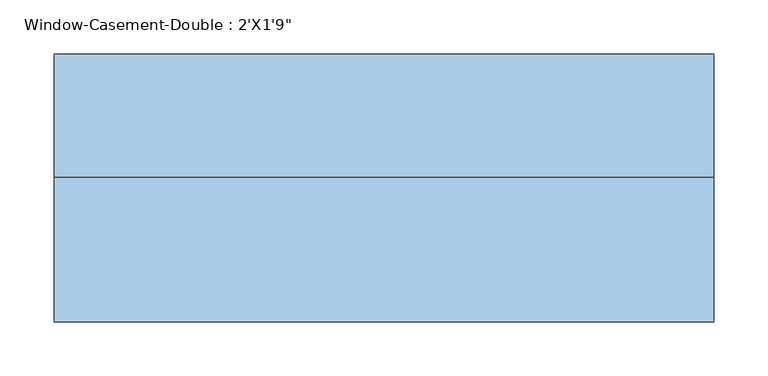
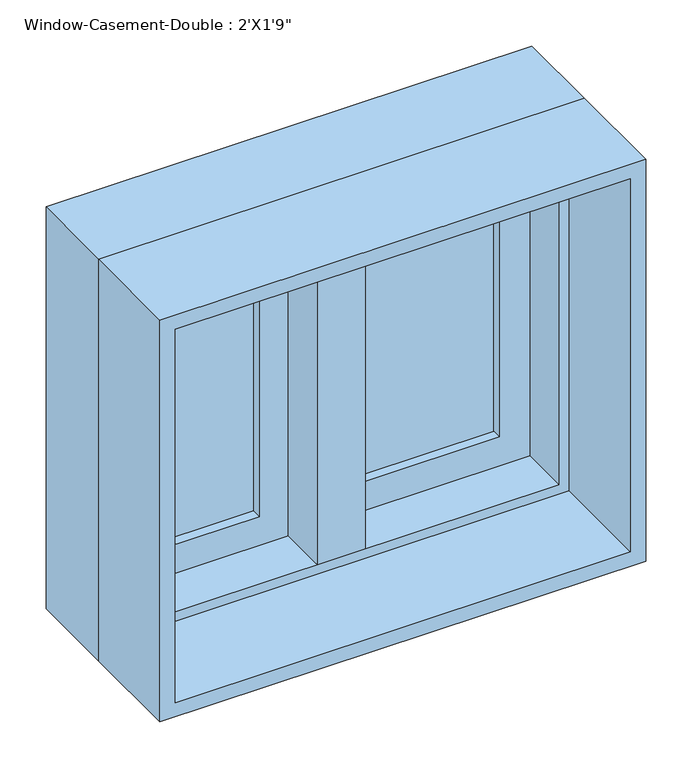
"""IFC4 building model written with IfcOpenShell, lengths in millimetres: window geometry."""

from ifc_helpers import new_model, si_unit, frame, origin, place, context, project, spatial, polyline, outline, extrude, faceted_brep, source, transform, mapped, element, save


def window_79894727(model_context):
    return source(origin(), model_context, "Body", "SolidModel", [
        faceted_brep([(9.525, 133.35, 2654.3), (-9.525, 133.35, 2654.3), (-9.525, 82.55, 2654.3), (9.525, 82.55, 2654.3), (9.525, 133.35, 2146.3), (9.525, 82.55, 2146.3), (-9.525, 82.55, 2146.3), (-9.525, 133.35, 2146.3), (-9.525, 82.55, 2165.35), (-9.525, 82.55, 2635.25), (-30.1625, 82.55, 2165.35), (-30.1625, 82.55, 2635.25), (-30.1625, 19.05, 2165.35), (-30.1625, 19.05, 2635.25), (30.1625, 19.05, 2165.35), (30.1625, 19.05, 2635.25), (30.1625, 82.55, 2165.35), (30.1625, 82.55, 2635.25), (9.525, 82.55, 2165.35), (9.525, 82.55, 2635.25)], [[[0, 1, 2, 3]], [[4, 5, 6, 7]], [[1, 0, 4, 7]], [[2, 1, 7, 6, 8, 9]], [[9, 8, 10, 11]], [[11, 10, 12, 13]], [[13, 12, 14, 15]], [[15, 14, 16, 17]], [[17, 16, 18, 19]], [[0, 3, 19, 18, 5, 4]], [[18, 8, 6, 5]], [[9, 19, 3, 2]], [[8, 18, 16, 14, 12, 10]], [[19, 9, 11, 13, 15, 17]]]),
        extrude(outline(polyline([(-66.675, 114.3), (-66.675, 107.95), (-234.95, 107.95), (-234.95, 114.3), (-66.675, 114.3)])), frame((0.0, 0.0, 2203.45), z_axis=(0.0, 0.0, 1.0), x_axis=(1.0, 0.0, 0.0)), (0.0, 0.0, 1.0), 393.7),
        extrude(outline(polyline([(-234.95, 95.25), (-234.95, 101.6), (-66.675, 101.6), (-66.675, 95.25), (-234.95, 95.25)])), frame((0.0, 0.0, 2203.45), z_axis=(0.0, 0.0, 1.0), x_axis=(1.0, 0.0, 0.0)), (0.0, 0.0, 1.0), 393.7),
        extrude(outline(polyline([(234.95, 114.3), (234.95, 107.95), (66.675, 107.95), (66.675, 114.3), (234.95, 114.3)])), frame((0.0, 0.0, 2203.45), z_axis=(0.0, 0.0, 1.0), x_axis=(1.0, 0.0, 0.0)), (0.0, 0.0, 1.0), 393.7),
        extrude(outline(polyline([(66.675, 95.25), (66.675, 101.6), (234.95, 101.6), (234.95, 95.25), (66.675, 95.25)])), frame((0.0, 0.0, 2203.45), z_axis=(0.0, 0.0, 1.0), x_axis=(1.0, 0.0, 0.0)), (0.0, 0.0, 1.0), 393.7),
        extrude(outline(polyline([(2654.3, -292.1), (2146.3, -292.1), (2146.3, -9.525), (2654.3, -9.525), (2654.3, -292.1)]), holes=[polyline([(2597.15, -66.675), (2203.45, -66.675), (2203.45, -234.95), (2597.15, -234.95), (2597.15, -66.675)])]), frame((0.0, 82.55, 0.0), z_axis=(0.0, 1.0, 0.0), x_axis=(0.0, 0.0, 1.0)), (0.0, 0.0, 1.0), 44.45),
        extrude(outline(polyline([(2146.3, 292.1), (2654.3, 292.1), (2654.3, 9.525), (2146.3, 9.525), (2146.3, 292.1)]), holes=[polyline([(2203.45, 66.675), (2597.15, 66.675), (2597.15, 234.95), (2203.45, 234.95), (2203.45, 66.675)])]), frame((0.0, 82.55, 0.0), z_axis=(0.0, 1.0, 0.0), x_axis=(0.0, 0.0, 1.0)), (0.0, 0.0, 1.0), 44.45),
        extrude(outline(polyline([(2667.0, -304.8), (2133.6, -304.8), (2133.6, 304.8), (2667.0, 304.8), (2667.0, -304.8)]), holes=[polyline([(2647.95, 285.75), (2152.65, 285.75), (2152.65, -285.75), (2647.95, -285.75), (2647.95, 285.75)])]), frame((0.0, -114.3, 0.0), z_axis=(0.0, 1.0, 0.0), x_axis=(0.0, 0.0, 1.0)), (0.0, 0.0, 1.0), 133.35),
        faceted_brep([(273.05, 82.55, 2635.25), (273.05, 19.05, 2635.25), (-273.05, 19.05, 2635.25), (-273.05, 82.55, 2635.25), (292.1, 133.35, 2654.3), (292.1, 82.55, 2654.3), (-292.1, 82.55, 2654.3), (-292.1, 133.35, 2654.3), (304.8, 19.05, 2667.0), (304.8, 133.35, 2667.0), (-304.8, 133.35, 2667.0), (-304.8, 19.05, 2667.0), (-273.05, 19.05, 2165.35), (-273.05, 82.55, 2165.35), (-292.1, 82.55, 2146.3), (-292.1, 133.35, 2146.3), (-304.8, 133.35, 2133.6), (-304.8, 19.05, 2133.6), (273.05, 19.05, 2165.35), (273.05, 82.55, 2165.35), (292.1, 82.55, 2146.3), (292.1, 133.35, 2146.3), (304.8, 133.35, 2133.6), (304.8, 19.05, 2133.6)], [[[0, 1, 2, 3]], [[4, 5, 6, 7]], [[8, 9, 10, 11]], [[3, 2, 12, 13]], [[7, 6, 14, 15]], [[11, 10, 16, 17]], [[13, 12, 18, 19]], [[15, 14, 20, 21]], [[17, 16, 22, 23]], [[11, 17, 23, 8], [1, 18, 12, 2]], [[19, 18, 1, 0]], [[5, 20, 14, 6], [3, 13, 19, 0]], [[21, 20, 5, 4]], [[23, 22, 9, 8]], [[9, 22, 16, 10], [7, 15, 21, 4]]]),
    ])


if __name__ == "__main__":
    model = new_model("IFC4")
    model_context = context("Model", 3, world=origin())
    ifc_project = project(units=[si_unit("LENGTHUNIT", "METRE", prefix="MILLI")], contexts=[model_context])
    site = spatial("IfcSite", under=ifc_project)
    building = spatial("IfcBuilding", under=site)
    placement = place(None, origin())
    window_shape = window_79894727(model_context)
    element("IfcWindow", 1, ObjectType="Window-Casement-Double : 2'X1'9\"", at=placement, inside=building, context=model_context, shape_type="MappedRepresentation", body=[
        mapped(window_shape, transform((0.0, 0.0, 0.0), x_axis=(1.0, 0.0, 0.0), y_axis=(0.0, 1.0, 0.0), z_axis=(0.0, 0.0, 1.0))),
    ])
    save(model, "model.ifc")

# Revit data of these elements
# Type "Window-Casement-Double : 2'X1'9\""
#   Type Mark = "22"
#   Fire Rating = "0.5h"
#   Assembly Code = "B2020100"
#   Analytic Construction = "Double glazing - domestic"
#   Frame Extension [instance default] = 0' - 0 1/4"
#   Window Inset [instance default] = 0' - 0"
#   Wall Thickness [instance default] = 0' - 6"
#   Interior Wall Closure [instance default] = 0' - 2 1/4"
#   Half Width = 1' - 0"
#   Visual Light Transmittance = 0.81
#   Thermal Resistance (R) = 1.8146 (h·ft²·°F)/BTU
#   Solar Heat Gain Coefficient = 0.76
#   Rough Width = 2' - 0 1/2"
#   Rough Height = 1' - 9 1/2"
#   Height = 1' - 9"
#   Heat Transfer Coefficient (U) = 0.5511 BTU/(h·ft²·°F)
#   Exterior Wall Closure [instance default] = 0' - 1 1/4"
#   Extension Jamb [instance default] = 0' - 2 1/4"
#   Default Sill Height = 7' - 0"
#   Width = 2' - 0"
#   Muntin Visibility = yes
#   Interior Trim Visibility [instance default] = yes
#   Exterior Trim Visibility [instance default] = yes
#   Extension Jamb Visibility [instance default] = yes
#   Interior Trim Material = Wood - Stained
#   Muntin Pattern = Muntin Pattern_2x2 : Muntin Pattern_2x2
#   Interior Trim = Trim-Window-Interior-Flat : Picture Frame
#   Interior Frame Material = Wood - Stained
#   Glass Panel Material = Glass
#   Exterior Trim Material = Clad - White
#   Exterior Trim = Trim-Window-Exterior-Flat : with Sill
#   Exterior Frame Material = Clad - White
#   Wall Closure = (empty or 0)
# Element 1 (IfcWindow, "Window-Casement-Double : 2'X1'9\"")
#   Wall Thickness = 0' - 9"
#   Extension Jamb = 0' - 5 1/4"
#   Materials on its faces: "Wood - Stained", "Glass", "Clad - White"
# Materials
#   "Wood - Stained": class "Wood", colour RGB 224 178 126, transparency 0, Cost = 0
#   "Glass": class "Glass", colour RGB 0 128 192, transparency 0.75, Description = "Soda Lime Glass", Cost = 0
#   "Clad - White": class "Wood", colour RGB 242 242 238, transparency 0, Cost = 0
